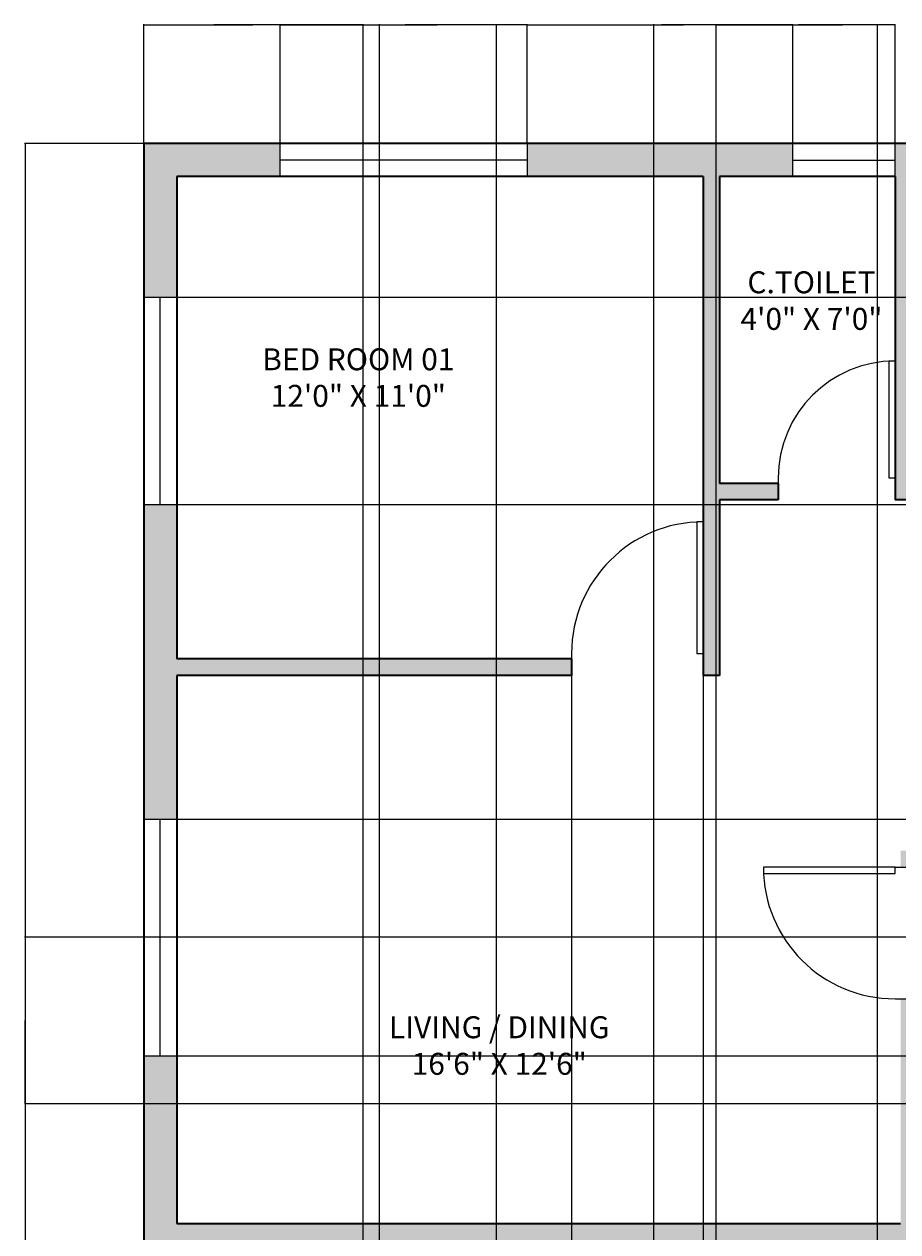
# Model space of a CAD drawing. Units: inches. Extents: x 2510 to 3056, y 673 to 1386.
# Tile 3 of 4: x 2510 to 2749, y 1056 to 1386. Entities that reach past the tile are written whole.
import ezdxf

# ---------------------------------------------------------------- set-up
doc = ezdxf.new("R2010")
doc.units = ezdxf.units.IN
for name, color, linetype, lineweight in [('A-ANNO-DIMS', 2, 'Continuous', 18), ('A-AREA-IDEN', 7, 'Continuous', 18), ('A-DOOR', 3, 'Continuous', 18), ('A-GLAZ', 4, 'Continuous', 18), ('A-WALL', 7, 'Continuous', 35), ('A-WALL-PATT', 252, 'Continuous', 13)]:
    doc.layers.add(name, color=color, linetype=linetype, lineweight=lineweight)
doc.styles.get("Standard").update_dxf_attribs({"font": 'arial.ttf'})
doc.dimstyles.get("Standard").update_dxf_attribs({"dimtxt": 0.18, "dimasz": 0.18, "dimexe": 0.18, "dimexo": 0.0625, "dimgap": 0.09, "dimtad": 0, "dimtih": 1, "dimtoh": 1, "dimdec": 4, "dimzin": 0, "dimdsep": 46, "dimtxsty": 'Standard', "dimcen": 0.09, "dimadec": 0, "dimazin": 0, "dimtfac": 1, "dimtdec": 4, "dimtofl": 0, "dimtmove": 0, "dimatfit": 3, "dimfxl": 1, "dimtolj": 1, "dimtzin": 0, "dimarcsym": 0})

# ---------------------------------------------------------------- blocks, each defined once
blk = doc.blocks.new('*U4')
for p, q in [((0, 0), (0, -6)), ((-36, 0), (-36, -6))]:
    blk.add_line(p, q)
blk.add_lwpolyline([(0, 0), (0, 36), (-1.75, 36), (-1.75, 0)], close=True)
blk.add_arc((0, 0), 36, 90, 180)
blk = doc.blocks.new('*U3')
for p, q in [((0, 0), (0, -6)), ((-32, 0), (-32, -6))]:
    blk.add_line(p, q)
blk.add_lwpolyline([(0, 0), (0, 32), (-1.75, 32), (-1.75, 0)], close=True)
blk.add_arc((0, 0), 32, 90, 180)
blk = doc.blocks.new('*D12')
at = {"layer": 'A-ANNO-DIMS', "color": 0, "lineweight": -2, "transparency": 16777216}
for p, q in [((2543.13, 1353.59), (2510.53, 1353.59)), ((2510.71, 1353.41), (2510.71, 1029.77)), ((2510.71, 705.77), (2510.71, 1029.4)), ((2543.13, 705.59), (2510.53, 705.59))]:
    blk.add_line(p, q, dxfattribs=at)
at = {"layer": 'A-ANNO-DIMS', "color": 0, "transparency": 16777216}
for points in [[(2510.68, 1353.41), (2510.74, 1353.41), (2510.71, 1353.59)], [(2510.68, 705.77), (2510.74, 705.77), (2510.71, 705.59)]]:
    blk.add_solid(points, dxfattribs=at)
at = {"layer": 'Defpoints', "color": 0, "transparency": 16777216}
for p in [(2510.71, 1353.59), (2543.19, 1353.59), (2543.19, 705.59)]:
    blk.add_point(p, dxfattribs=at)
at = {"layer": 'A-ANNO-DIMS', "color": 0, "transparency": 16777216, "insert": (2510.71, 1029.59), "char_height": 0.18, "attachment_point": 5}
blk.add_mtext('\\A1;648', dxfattribs=at)
blk = doc.blocks.new('*D14')
at = {"layer": 'A-ANNO-DIMS', "color": 0, "lineweight": -2, "transparency": 16777216}
for p, q in [((2543.19, 1353.65), (2543.19, 1386.25)), ((2543.37, 1386.07), (2561.39, 1386.07)), ((2580.34, 1386.07), (2562.32, 1386.07)), ((2580.52, 1353.65), (2580.52, 1386.25))]:
    blk.add_line(p, q, dxfattribs=at)
at = {"layer": 'A-ANNO-DIMS', "color": 0, "transparency": 16777216}
for points in [[(2543.37, 1386.1), (2543.37, 1386.04), (2543.19, 1386.07)], [(2580.34, 1386.1), (2580.34, 1386.04), (2580.52, 1386.07)]]:
    blk.add_solid(points, dxfattribs=at)
at = {"layer": 'Defpoints', "color": 0, "transparency": 16777216}
for p in [(2580.52, 1386.07), (2543.19, 1353.59), (2580.52, 1353.59)]:
    blk.add_point(p, dxfattribs=at)
at = {"layer": 'A-ANNO-DIMS', "color": 0, "transparency": 16777216, "insert": (2561.85, 1386.07), "char_height": 0.18, "attachment_point": 5}
blk.add_mtext('\\A1;37.324', dxfattribs=at)
blk = doc.blocks.new('*D15')
at = {"layer": 'A-ANNO-DIMS', "color": 0, "lineweight": -2, "transparency": 16777216}
for p, q in [((2580.52, 1353.65), (2580.52, 1386.25)), ((2580.7, 1386.07), (2613.89, 1386.07)), ((2647.87, 1386.07), (2614.68, 1386.07)), ((2648.05, 1353.65), (2648.05, 1386.25))]:
    blk.add_line(p, q, dxfattribs=at)
at = {"layer": 'A-ANNO-DIMS', "color": 0, "transparency": 16777216}
for points in [[(2580.7, 1386.1), (2580.7, 1386.04), (2580.52, 1386.07)], [(2647.87, 1386.1), (2647.87, 1386.04), (2648.05, 1386.07)]]:
    blk.add_solid(points, dxfattribs=at)
at = {"layer": 'Defpoints', "color": 0, "transparency": 16777216}
for p in [(2648.05, 1386.07), (2580.52, 1353.59), (2648.05, 1353.59)]:
    blk.add_point(p, dxfattribs=at)
at = {"layer": 'A-ANNO-DIMS', "color": 0, "transparency": 16777216, "insert": (2614.28, 1386.07), "char_height": 0.18, "attachment_point": 5}
blk.add_mtext('\\A1;67.53', dxfattribs=at)
blk = doc.blocks.new('*D16')
at = {"layer": 'A-ANNO-DIMS', "color": 0, "lineweight": -2, "transparency": 16777216}
for p, q in [((2648.05, 1353.65), (2648.05, 1386.25)), ((2648.23, 1386.07), (2683.99, 1386.07)), ((2720.53, 1386.07), (2684.77, 1386.07)), ((2720.71, 1353.65), (2720.71, 1386.25))]:
    blk.add_line(p, q, dxfattribs=at)
at = {"layer": 'A-ANNO-DIMS', "color": 0, "transparency": 16777216}
for points in [[(2648.23, 1386.1), (2648.23, 1386.04), (2648.05, 1386.07)], [(2720.53, 1386.1), (2720.53, 1386.04), (2720.71, 1386.07)]]:
    blk.add_solid(points, dxfattribs=at)
at = {"layer": 'Defpoints', "color": 0, "transparency": 16777216}
for p in [(2720.71, 1386.07), (2648.05, 1353.59), (2720.71, 1353.59)]:
    blk.add_point(p, dxfattribs=at)
at = {"layer": 'A-ANNO-DIMS', "color": 0, "transparency": 16777216, "insert": (2684.38, 1386.07), "char_height": 0.18, "attachment_point": 5}
blk.add_mtext('\\A1;72.66', dxfattribs=at)
blk = doc.blocks.new('*D17')
at = {"layer": 'A-ANNO-DIMS', "color": 0, "lineweight": -2, "transparency": 16777216}
for p, q in [((2720.71, 1353.65), (2720.71, 1386.25)), ((2720.89, 1386.07), (2734.31, 1386.07)), ((2748.51, 1386.07), (2735.1, 1386.07)), ((2748.69, 1353.65), (2748.69, 1386.25))]:
    blk.add_line(p, q, dxfattribs=at)
at = {"layer": 'A-ANNO-DIMS', "color": 0, "transparency": 16777216}
for points in [[(2720.89, 1386.1), (2720.89, 1386.04), (2720.71, 1386.07)], [(2748.51, 1386.1), (2748.51, 1386.04), (2748.69, 1386.07)]]:
    blk.add_solid(points, dxfattribs=at)
at = {"layer": 'Defpoints', "color": 0, "transparency": 16777216}
for p in [(2748.69, 1386.07), (2720.71, 1353.59), (2748.69, 1353.59)]:
    blk.add_point(p, dxfattribs=at)
at = {"layer": 'A-ANNO-DIMS', "color": 0, "transparency": 16777216, "insert": (2734.7, 1386.07), "char_height": 0.18, "attachment_point": 5}
blk.add_mtext('\\A1;27.98', dxfattribs=at)
blk = doc.blocks.new('*D32')
at = {"layer": 'A-ANNO-DIMS', "color": 0, "lineweight": -2, "transparency": 16777216}
for p, q in [((3014.13, 1136.48), (2510.53, 1136.48)), ((2510.71, 1136.3), (2510.71, 1113.86)), ((2510.71, 1091.06), (2510.71, 1113.5)), ((3014.13, 1090.88), (2510.53, 1090.88))]:
    blk.add_line(p, q, dxfattribs=at)
at = {"layer": 'A-ANNO-DIMS', "color": 0, "transparency": 16777216}
for points in [[(2510.68, 1136.3), (2510.74, 1136.3), (2510.71, 1136.48)], [(2510.68, 1091.06), (2510.74, 1091.06), (2510.71, 1090.88)]]:
    blk.add_solid(points, dxfattribs=at)
at = {"layer": 'Defpoints', "color": 0, "transparency": 16777216}
for p in [(2510.71, 1136.48), (3014.19, 1136.48), (3014.19, 1090.88)]:
    blk.add_point(p, dxfattribs=at)
at = {"layer": 'A-ANNO-DIMS', "color": 0, "transparency": 16777216, "insert": (2510.71, 1113.68), "char_height": 0.18, "attachment_point": 5}
blk.add_mtext('\\A1;45.6', dxfattribs=at)
blk = doc.blocks.new('*D36')
at = {"layer": 'A-ANNO-DIMS', "color": 0, "lineweight": -2, "transparency": 16777216}
for p, q in [((2552.25, 1168.75), (3055.85, 1168.75)), ((3055.67, 1168.57), (3055.67, 1136.56)), ((3055.67, 1104.19), (3055.67, 1136.2)), ((2552.25, 1104.01), (3055.85, 1104.01))]:
    blk.add_line(p, q, dxfattribs=at)
at = {"layer": 'A-ANNO-DIMS', "color": 0, "transparency": 16777216}
for points in [[(3055.64, 1168.57), (3055.7, 1168.57), (3055.67, 1168.75)], [(3055.64, 1104.19), (3055.7, 1104.19), (3055.67, 1104.01)]]:
    blk.add_solid(points, dxfattribs=at)
at = {"layer": 'Defpoints', "color": 0, "transparency": 16777216}
for p in [(2552.19, 1168.75), (3055.67, 1168.75), (2552.19, 1104.01)]:
    blk.add_point(p, dxfattribs=at)
at = {"layer": 'A-ANNO-DIMS', "color": 0, "transparency": 16777216, "insert": (3055.67, 1136.38), "char_height": 0.18, "attachment_point": 5}
blk.add_mtext('\\A1;64.74', dxfattribs=at)
blk = doc.blocks.new('*D37')
at = {"layer": 'A-ANNO-DIMS', "color": 0, "lineweight": -2, "transparency": 16777216}
for p, q in [((2552.25, 1311.56), (3055.85, 1311.56)), ((3055.67, 1311.38), (3055.67, 1283.38)), ((3055.67, 1255.02), (3055.67, 1283.02)), ((2552.25, 1254.84), (3055.85, 1254.84))]:
    blk.add_line(p, q, dxfattribs=at)
at = {"layer": 'A-ANNO-DIMS', "color": 0, "transparency": 16777216}
for points in [[(3055.64, 1311.38), (3055.7, 1311.38), (3055.67, 1311.56)], [(3055.64, 1255.02), (3055.7, 1255.02), (3055.67, 1254.84)]]:
    blk.add_solid(points, dxfattribs=at)
at = {"layer": 'Defpoints', "color": 0, "transparency": 16777216}
for p in [(2552.19, 1311.56), (3055.67, 1311.56), (2552.19, 1254.84)]:
    blk.add_point(p, dxfattribs=at)
at = {"layer": 'A-ANNO-DIMS', "color": 0, "transparency": 16777216, "insert": (3055.67, 1283.2), "char_height": 0.18, "attachment_point": 5}
blk.add_mtext('\\A1;56.72', dxfattribs=at)
blk = doc.blocks.new('*D40')
at = {"layer": 'A-ANNO-DIMS', "color": 0, "lineweight": -2, "transparency": 16777216}
for p, q in [((2682.69, 719.15), (2682.69, 1386.25)), ((2682.87, 1386.07), (2690.76, 1386.07)), ((2699.56, 1386.07), (2691.67, 1386.07)), ((2699.74, 719.15), (2699.74, 1386.25))]:
    blk.add_line(p, q, dxfattribs=at)
at = {"layer": 'A-ANNO-DIMS', "color": 0, "transparency": 16777216}
for points in [[(2682.87, 1386.1), (2682.87, 1386.04), (2682.69, 1386.07)], [(2699.56, 1386.1), (2699.56, 1386.04), (2699.74, 1386.07)]]:
    blk.add_solid(points, dxfattribs=at)
at = {"layer": 'Defpoints', "color": 0, "transparency": 16777216}
for p in [(2699.74, 1386.07), (2682.69, 719.09), (2699.74, 719.09)]:
    blk.add_point(p, dxfattribs=at)
at = {"layer": 'A-ANNO-DIMS', "color": 0, "transparency": 16777216, "insert": (2691.22, 1386.07), "char_height": 0.18, "attachment_point": 5}
blk.add_mtext('\\A1;17.045', dxfattribs=at)
blk = doc.blocks.new('*D41')
at = {"layer": 'A-ANNO-DIMS', "color": 0, "lineweight": -2, "transparency": 16777216}
for p, q in [((2699.74, 719.15), (2699.74, 1386.25)), ((2699.92, 1386.07), (2721.41, 1386.07)), ((2743.7, 1386.07), (2722.21, 1386.07)), ((2743.88, 719.15), (2743.88, 1386.25))]:
    blk.add_line(p, q, dxfattribs=at)
at = {"layer": 'A-ANNO-DIMS', "color": 0, "transparency": 16777216}
for points in [[(2699.92, 1386.1), (2699.92, 1386.04), (2699.74, 1386.07)], [(2743.7, 1386.1), (2743.7, 1386.04), (2743.88, 1386.07)]]:
    blk.add_solid(points, dxfattribs=at)
at = {"layer": 'Defpoints', "color": 0, "transparency": 16777216}
for p in [(2743.88, 1386.07), (2699.74, 719.09), (2743.88, 719.09)]:
    blk.add_point(p, dxfattribs=at)
at = {"layer": 'A-ANNO-DIMS', "color": 0, "transparency": 16777216, "insert": (2721.81, 1386.07), "char_height": 0.18, "attachment_point": 5}
blk.add_mtext('\\A1;44.14', dxfattribs=at)
blk = doc.blocks.new('*D45')
at = {"layer": 'A-ANNO-DIMS', "color": 0, "lineweight": -2, "transparency": 16777216}
for p, q in [((2660.19, 1208.02), (2660.19, 672.93)), ((2696.19, 1208.02), (2696.19, 672.93)), ((2660.37, 673.11), (2677.97, 673.11)), ((2696.01, 673.11), (2678.41, 673.11))]:
    blk.add_line(p, q, dxfattribs=at)
at = {"layer": 'A-ANNO-DIMS', "color": 0, "transparency": 16777216}
for points in [[(2660.37, 673.14), (2660.37, 673.08), (2660.19, 673.11)], [(2696.01, 673.14), (2696.01, 673.08), (2696.19, 673.11)]]:
    blk.add_solid(points, dxfattribs=at)
at = {"layer": 'Defpoints', "color": 0, "transparency": 16777216}
for p in [(2660.19, 1208.09), (2696.19, 1208.09), (2696.19, 673.11)]:
    blk.add_point(p, dxfattribs=at)
at = {"layer": 'A-ANNO-DIMS', "color": 0, "transparency": 16777216, "insert": (2678.19, 673.11), "char_height": 0.18, "attachment_point": 5}
blk.add_mtext('\\A1;36', dxfattribs=at)
blk = doc.blocks.new('*D50')
at = {"layer": 'A-ANNO-DIMS', "color": 0, "lineweight": -2, "transparency": 16777216}
for p, q in [((2607.69, 750.65), (2607.69, 1386.25)), ((2607.87, 1386.07), (2623.47, 1386.07)), ((2639.51, 1386.07), (2623.91, 1386.07)), ((2639.69, 750.65), (2639.69, 1386.25))]:
    blk.add_line(p, q, dxfattribs=at)
at = {"layer": 'A-ANNO-DIMS', "color": 0, "transparency": 16777216}
for points in [[(2607.87, 1386.1), (2607.87, 1386.04), (2607.69, 1386.07)], [(2639.51, 1386.1), (2639.51, 1386.04), (2639.69, 1386.07)]]:
    blk.add_solid(points, dxfattribs=at)
at = {"layer": 'Defpoints', "color": 0, "transparency": 16777216}
for p in [(2639.69, 1386.07), (2607.69, 750.59), (2639.69, 750.59)]:
    blk.add_point(p, dxfattribs=at)
at = {"layer": 'A-ANNO-DIMS', "color": 0, "transparency": 16777216, "insert": (2623.69, 1386.07), "char_height": 0.18, "attachment_point": 5}
blk.add_mtext('\\A1;32', dxfattribs=at)
blk = doc.blocks.new('*D57')
at = {"layer": 'A-ANNO-DIMS', "color": 0, "lineweight": -2, "transparency": 16777216}
for p, q in [((2543.19, 705.65), (2543.19, 1386.25)), ((2543.37, 1386.07), (2572.97, 1386.07)), ((2603.01, 1386.07), (2573.41, 1386.07)), ((2603.19, 705.65), (2603.19, 1386.25))]:
    blk.add_line(p, q, dxfattribs=at)
at = {"layer": 'A-ANNO-DIMS', "color": 0, "transparency": 16777216}
for points in [[(2543.37, 1386.1), (2543.37, 1386.04), (2543.19, 1386.07)], [(2603.01, 1386.1), (2603.01, 1386.04), (2603.19, 1386.07)]]:
    blk.add_solid(points, dxfattribs=at)
at = {"layer": 'Defpoints', "color": 0, "transparency": 16777216}
for p in [(2603.19, 1386.07), (2543.19, 705.59), (2603.19, 705.59)]:
    blk.add_point(p, dxfattribs=at)
at = {"layer": 'A-ANNO-DIMS', "color": 0, "transparency": 16777216, "insert": (2573.19, 1386.07), "char_height": 0.18, "attachment_point": 5}
blk.add_mtext('\\A1;60', dxfattribs=at)

msp = doc.modelspace()

# ---------------------------------------------------------------- hatches: boundary and pattern name
at = {"layer": 'A-WALL-PATT'}
h = msp.add_hatch(color=256, dxfattribs=at)
h.dxf.hatch_style = 1
h.paths.add_polyline_path([(2580.5162, 1353.5862), (2543.1924, 1353.5862), (2543.1924, 1311.5591), (2552.1924, 1311.5591), (2552.1924, 1344.5862), (2580.5162, 1344.5862)])
h.paths.add_polyline_path([(2720.7125, 1353.5862), (2648.0497, 1353.5862), (2648.0497, 1344.5862), (2696.1924, 1344.5862), (2696.1924, 1208.0862), (2700.6924, 1208.0862), (2700.6924, 1256.0862), (2716.6924, 1256.0862), (2716.6924, 1260.5862), (2700.6924, 1260.5862), (2700.6924, 1344.5862), (2720.7125, 1344.5862)])
h.paths.add_polyline_path([(2762.4727, 1353.5862), (2748.6924, 1353.5862), (2748.6924, 1344.5862), (2748.6924, 1256.0862), (2753.1924, 1256.0862), (2753.1924, 1262.0862), (2753.1924, 1294.0862), (2753.1924, 1344.5862), (2762.4727, 1344.5862)])
h.paths.add_polyline_path([(2863.5016, 1353.5862), (2808.6621, 1353.5862), (2808.6621, 1344.5862), (2825.1924, 1344.5862), (2825.1924, 1260.5862), (2785.1924, 1260.5862), (2785.1924, 1256.0862), (2825.1924, 1256.0862), (2825.1924, 1248.5862), (2829.6924, 1248.5862), (2829.6924, 1344.5862), (2863.5016, 1344.5862)])
h.paths.add_polyline_path([(2966.1924, 1353.5862), (2915.7284, 1353.5862), (2915.7284, 1344.5862), (2961.6924, 1344.5862), (2961.6924, 1212.5862), (2897.6924, 1212.5862), (2897.6924, 1208.0862), (2961.6924, 1208.0862), (2961.6924, 1193.4346), (2966.1924, 1193.4346), (2966.1924, 1208.0862)])
h.paths.add_polyline_path([(2660.1924, 1212.5862), (2552.1924, 1212.5862), (2552.1924, 1254.8401), (2543.1924, 1254.8401), (2543.1924, 1168.7504), (2552.1924, 1168.7504), (2552.1924, 1208.0862), (2660.1924, 1208.0862)])
h.paths.add_polyline_path([(3023.1924, 1160.0862), (2966.1924, 1160.0862), (2966.1924, 1165.033), (2961.6924, 1165.033), (2961.6924, 1160.0862), (2865.6924, 1160.0862), (2865.6924, 1212.5862), (2825.1924, 1212.5862), (2825.1924, 1208.0862), (2861.1924, 1208.0862), (2861.1924, 1160.0862), (2750.1527, 1160.0862), (2750.1527, 1155.5862), (2754.6527, 1155.5862), (2966.1924, 1155.5862), (3014.1924, 1155.5862), (3014.1924, 1136.4806), (3023.1924, 1136.4806)])
h.paths.add_polyline_path([(3023.1924, 1090.8839), (3014.1924, 1090.8839), (3014.1924, 1058.0862), (2807.1924, 1058.0862), (2807.1924, 1053.5862), (2879.1924, 1053.5862), (2879.1924, 929.0862), (2883.6924, 929.0862), (2883.6924, 935.0862), (2883.6924, 971.0862), (2883.6924, 1053.5862), (3014.1924, 1053.5862), (3014.1924, 1028.0329), (3023.1924, 1028.0329)])
h.paths.add_polyline_path([(3023.1924, 970.6943), (3014.1924, 970.6943), (3014.1924, 933.5862), (2919.6924, 933.5862), (2919.6924, 929.0862), (2927.1924, 929.0862), (2927.1924, 907.0862), (2931.6924, 907.0862), (2931.6924, 929.0862), (3014.1924, 929.0862), (3014.1924, 918.5377), (3023.1924, 918.5377)])
h.paths.add_polyline_path([(3023.1924, 886.219), (3014.1924, 886.219), (3014.1924, 875.0862), (2927.1924, 875.0862), (2879.1924, 875.0862), (2879.1924, 870.5862), (2885.1924, 870.5862), (2921.1924, 870.5862), (3014.1924, 870.5862), (3014.1924, 835.4806), (3023.1924, 835.4806)])
h.paths.add_polyline_path([(3023.1924, 775.6299), (3014.1924, 775.6299), (3014.1924, 746.0862), (3023.1924, 746.0862)])
h.paths.add_polyline_path([(2958.6924, 750.5862), (2954.1924, 750.5862), (2954.1924, 744.5862), (2954.1924, 716.5862), (2954.1924, 710.0862), (2910.6841, 710.0862), (2910.6841, 705.5862), (2958.6924, 705.5862)])
h.paths.add_polyline_path([(2926.1924, 750.5862), (2883.6924, 750.5862), (2883.6924, 834.5862), (2879.1924, 834.5862), (2879.1924, 819.5862), (2815.1924, 819.5862), (2815.1924, 815.0862), (2879.1924, 815.0862), (2879.1924, 746.0862), (2879.1924, 719.0862), (2862.8388, 719.0862), (2862.8388, 714.5862), (2879.1924, 714.5862), (2879.1924, 705.5862), (2883.6924, 705.5862), (2883.6924, 710.0862), (2883.6924, 746.0862), (2926.1924, 746.1758)])
h.paths.add_polyline_path([(2682.6924, 815.0862), (2746.6924, 815.0862), (2746.6924, 819.5862), (2682.6924, 819.5862), (2682.6924, 834.5862), (2678.1924, 834.5862), (2678.1924, 750.5862), (2639.6924, 750.5862), (2639.6924, 746.0862), (2678.1924, 746.0862), (2678.1924, 710.0862), (2678.1924, 705.5862), (2682.6924, 705.5862), (2682.6924, 714.5862), (2699.7376, 714.5862), (2699.7376, 719.0862), (2682.6924, 719.0862), (2682.6924, 746.0862)])
h.paths.add_polyline_path([(2650.2761, 710.0862), (2607.6924, 710.0862), (2607.6924, 750.5862), (2603.1924, 750.5862), (2603.1924, 705.5862), (2607.6924, 705.5862), (2650.2761, 705.5862)])
h.paths.add_polyline_path([(2552.1924, 777.7158), (2543.1924, 777.7158), (2543.1924, 746.0862), (2552.1924, 746.0862)])
h.paths.add_polyline_path([(2828.3093, 719.0862), (2783.1924, 719.0862), (2783.1924, 815.0862), (2783.1924, 1058.0862), (2778.6924, 1058.0862), (2778.6924, 815.0862), (2778.6924, 719.0862), (2743.8813, 719.0862), (2743.8813, 714.5862), (2778.6924, 714.5862), (2828.3093, 714.5862)])
h.paths.add_polyline_path([(2642.1924, 933.5862), (2552.1924, 933.5862), (2552.1924, 965.3494), (2543.1924, 965.3494), (2543.1924, 907.809), (2552.1924, 907.809), (2552.1924, 929.0862), (2630.1924, 929.0862), (2630.1924, 907.0862), (2634.6924, 907.0862), (2634.6924, 929.0862), (2642.1924, 929.0862)])
h.paths.add_polyline_path([(2682.6924, 875.0862), (2552.1924, 875.0862), (2543.1924, 875.0862), (2543.1924, 832.3664), (2552.1924, 832.3664), (2552.1924, 870.5862), (2634.6924, 870.5862), (2682.6924, 870.5862)])
h.paths.add_polyline_path([(2754.6527, 1119.5862), (2750.1527, 1119.5862), (2750.1527, 1058.0862), (2552.1924, 1058.0862), (2552.1924, 1104.0128), (2543.1924, 1104.0128), (2543.1924, 1017.3235), (2552.1924, 1017.3235), (2552.1924, 1053.5862), (2678.1924, 1053.5862), (2678.1924, 929.0862), (2682.6924, 929.0862), (2682.6924, 1053.5862), (2754.6527, 1053.5862)])

# ---------------------------------------------------------------- linework, layer by layer
at = {"layer": 'A-GLAZ'}
for p, q in [((2580.5162, 1344.5862), (2580.5162, 1353.5862)), ((2648.0497, 1353.5862), (2648.0497, 1344.5862)), ((2720.7125, 1344.5529), (2720.7125, 1353.5862)), ((2748.6924, 1344.5862), (2748.6924, 1353.5862)), ((2580.5162, 1349.0862), (2648.0497, 1349.0862)), ((2720.7125, 1349.0695), (2748.6924, 1349.0695)), ((2543.1924, 1311.5591), (2552.1924, 1311.5591)), ((2547.6924, 1254.8401), (2547.6924, 1311.5591)), ((2543.1924, 1254.8401), (2552.1924, 1254.8401)), ((2543.1924, 1168.7504), (2552.1924, 1168.7504)), ((2547.6924, 1104.0128), (2547.6924, 1168.7504)), ((2543.1924, 1104.0128), (2552.1924, 1104.0128))]:
    msp.add_line(p, q, dxfattribs=at)
at = {"layer": 'A-WALL'}
for p, q in [((2966.1924, 1353.5862), (2543.1924, 1353.5862)), ((2543.1924, 1353.5862), (2543.1924, 705.5862)), ((2552.1924, 1344.5862), (2552.1924, 1212.5862)), ((2696.1924, 1344.5862), (2552.1924, 1344.5862)), ((2696.1924, 1344.5862), (2696.1924, 1208.0862)), ((2700.6924, 1344.5862), (2700.6924, 1260.5862)), ((2748.6924, 1344.5862), (2700.6924, 1344.5862)), ((2748.6924, 1344.5862), (2748.6924, 1256.0862)), ((2716.6924, 1260.5862), (2700.6924, 1260.5862)), ((2716.6924, 1260.5862), (2716.6924, 1256.0862)), ((2716.6924, 1256.0862), (2700.6924, 1256.0862)), ((2700.6924, 1256.0862), (2700.6924, 1208.0862)), ((2753.1924, 1256.0862), (2748.6924, 1256.0862)), ((2660.1924, 1212.5862), (2552.1924, 1212.5862)), ((2660.1924, 1212.5862), (2660.1924, 1208.0862)), ((2552.1924, 1208.0862), (2552.1924, 1058.0862)), ((2660.1924, 1208.0862), (2552.1924, 1208.0862)), ((2700.6924, 1208.0862), (2696.1924, 1208.0862)), ((2552.1924, 1058.0862), (2750.1527, 1058.0862))]:
    msp.add_line(p, q, dxfattribs=at)

# ---------------------------------------------------------------- block references
at = {"layer": 'A-DOOR'}
for name, p in [('*U3', (2748.6924, 1262.0862)), ('*U4', (2696.1924, 1214.0862))]:
    msp.add_blockref(name, p, dxfattribs=at)
at = {"layer": 'A-DOOR', "rotation": 90}
msp.add_blockref('*U4', (2748.6527, 1155.5862), dxfattribs=at)

# ---------------------------------------------------------------- texts
at = {"layer": 'A-AREA-IDEN', "char_height": 6, "attachment_point": 1}
for s, width, insert in [('\\pxqc;C.TOILET\\P4\'0" X 7\'0"', 59.569763, (2696.0186, 1318.6131)), ('\\pxqc;BED ROOM 01\\P12\'0" X 11\'0"', 59.569763, (2572.0833, 1297.5557)), ('\\pxqc;LIVING / DINING\\P16\'6" X 12\'6"', 65.599533, (2607.613, 1114.8062))]:
    msp.add_mtext_dynamic_manual_height_columns(s, width=width, gutter_width=12.5, heights=[0], dxfattribs=dict(at, insert=insert))

# ---------------------------------------------------------------- dimensions: what is measured, and where the dimension line sits
at = {"layer": 'A-ANNO-DIMS'}
for base, p1, p2, override, picture, middle in [((2580.5162, 1386.0667), (2543.1924, 1353.5862), (2580.5162, 1353.5862), {"dimdec": 3, "dimlfac": 1, "dimrnd": 0, "dimzin": 0, "dimdsep": 46, "dimlunit": 2}, '*D14', (2561.8543, 1386.0667)), ((2603.1924, 1386.0667), (2543.1924, 705.5862), (2603.1924, 705.5862), {"dimdec": 0, "dimlfac": 1, "dimrnd": 0, "dimzin": 0, "dimdsep": 46, "dimlunit": 2}, '*D57', (2573.1924, 1386.0667)), ((2648.0497, 1386.0667), (2580.5162, 1353.5862), (2648.0497, 1353.5862), {"dimdec": 2, "dimlfac": 1, "dimrnd": 0, "dimzin": 0, "dimdsep": 46, "dimlunit": 2}, '*D15', (2614.283, 1386.0667)), ((2639.6924, 1386.0667), (2607.6924, 750.5862), (2639.6924, 750.5862), {"dimdec": 0, "dimlfac": 1, "dimrnd": 0, "dimzin": 0, "dimdsep": 46, "dimlunit": 2}, '*D50', (2623.6924, 1386.0667)), ((2720.7125, 1386.0667), (2648.0497, 1353.5862), (2720.7125, 1353.5862), {"dimdec": 2, "dimlfac": 1, "dimrnd": 0, "dimzin": 0, "dimdsep": 46, "dimlunit": 2}, '*D16', (2684.3811, 1386.0667)), ((2699.7376, 1386.0667), (2682.6924, 719.0862), (2699.7376, 719.0862), {"dimdec": 3, "dimlfac": 1, "dimrnd": 0, "dimzin": 0, "dimdsep": 46, "dimlunit": 2}, '*D40', (2691.215, 1386.0667)), ((2743.8813, 1386.0667), (2699.7376, 719.0862), (2743.8813, 719.0862), {"dimdec": 2, "dimlfac": 1, "dimrnd": 0, "dimzin": 0, "dimdsep": 46, "dimlunit": 2}, '*D41', (2721.8095, 1386.0667)), ((2748.6924, 1386.0667), (2720.7125, 1353.5862), (2748.6924, 1353.5862), {"dimdec": 2, "dimlfac": 1, "dimrnd": 0, "dimzin": 0, "dimdsep": 46, "dimlunit": 2}, '*D17', (2734.7025, 1386.0667)), ((2696.1924, 673.1057), (2660.1924, 1208.0862), (2696.1924, 1208.0862), {"dimdec": 0, "dimlfac": 1, "dimrnd": 0, "dimzin": 0, "dimdsep": 46, "dimlunit": 2}, '*D45', (2678.1924, 673.1057))]:
    dim = msp.add_linear_dim(base=base, p1=p1, p2=p2, dimstyle='Standard', override=override, dxfattribs=at)
    dim.commit()
    dim.dimension.update_dxf_attribs({"geometry": picture, "text_midpoint": middle})
for base, p1, p2, override, picture, middle in [((2510.7119, 1353.5862), (2543.1924, 705.5862), (2543.1924, 1353.5862), {"dimdec": 0, "dimlfac": 1, "dimrnd": 0, "dimzin": 0, "dimdsep": 46, "dimlunit": 2}, '*D12', (2510.7119, 1029.5862)), ((3055.6729, 1311.5591), (2552.1924, 1254.8401), (2552.1924, 1311.5591), {"dimdec": 2, "dimlfac": 1, "dimrnd": 0, "dimzin": 0, "dimdsep": 46, "dimlunit": 2}, '*D37', (3055.6729, 1283.1996)), ((3055.6729, 1168.7504), (2552.1924, 1104.0128), (2552.1924, 1168.7504), {"dimdec": 2, "dimlfac": 1, "dimrnd": 0, "dimzin": 0, "dimdsep": 46, "dimlunit": 2}, '*D36', (3055.6729, 1136.3816)), ((2510.7119, 1136.4806), (3014.1924, 1090.8839), (3014.1924, 1136.4806), {"dimdec": 1, "dimlfac": 1, "dimrnd": 0, "dimzin": 0, "dimdsep": 46, "dimlunit": 2}, '*D32', (2510.7119, 1113.6823))]:
    dim = msp.add_linear_dim(base=base, p1=p1, p2=p2, angle=90, dimstyle='Standard', override=override, dxfattribs=at)
    dim.commit()
    dim.dimension.update_dxf_attribs({"geometry": picture, "text_midpoint": middle})

doc.saveas('drawing.dxf')
